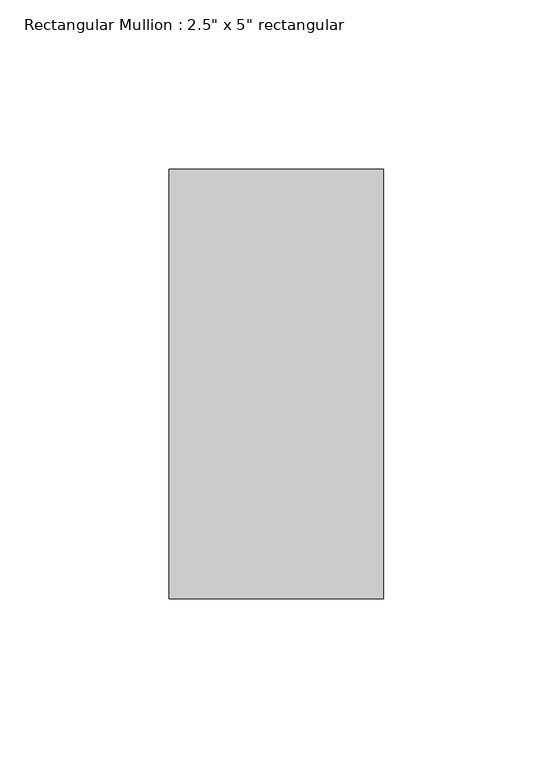
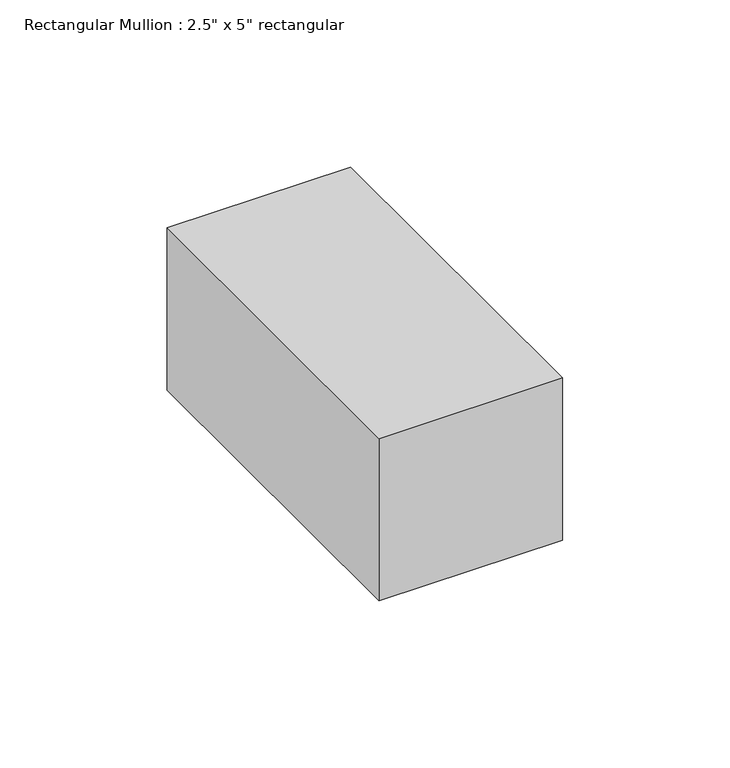
"""IFC4 building model written with IfcOpenShell, lengths in millimetres: member geometry."""

from ifc_helpers import new_model, si_unit, frame, origin, place, context, project, spatial, polyline, outline, extrude, source, transform, mapped, element, save


def member_4557678a(model_context):
    return source(origin(), model_context, "Body", "SweptSolid", [
        extrude(outline(polyline([(31.75, 63.5), (31.75, -63.5), (-31.75, -63.5), (-31.75, 63.5), (31.75, 63.5)])), frame((0.0, 0.0, -59.2666667), z_axis=(0.0, 0.0, 1.0), x_axis=(1.0, 0.0, 0.0)), (0.0, 0.0, 1.0), 59.2666667),
    ])


if __name__ == "__main__":
    model = new_model("IFC4")
    model_context = context("Model", 3, world=origin())
    ifc_project = project(units=[si_unit("LENGTHUNIT", "METRE", prefix="MILLI")], contexts=[model_context])
    site = spatial("IfcSite", under=ifc_project)
    building = spatial("IfcBuilding", under=site)
    placement = place(None, origin())
    member_shape = member_4557678a(model_context)
    element("IfcMember", 1, ObjectType="Rectangular Mullion : 2.5\" x 5\" rectangular", at=placement, inside=building, context=model_context, shape_type="MappedRepresentation", body=[
        mapped(member_shape, transform((0.0, 0.0, 0.0), x_axis=(1.0, 0.0, 0.0), y_axis=(0.0, 1.0, 0.0), z_axis=(0.0, 0.0, 1.0))),
    ])
    save(model, "model.ifc")

# Revit data of these elements
# Type "Rectangular Mullion : 2.5\" x 5\" rectangular"
#   built-in parameter 1007304 = 0.416667 (stored number, unit not read)
#   built-in parameter 1007301 = 0.104167 (stored number, unit not read)
#   built-in parameter 1007300 = 0.104167 (stored number, unit not read)
# Element 1 (IfcMember, "Rectangular Mullion : 2.5\" x 5\" rectangular")
#   Materials on its faces: "Aluminum"
# Materials
#   "Aluminum": class "Metal", colour RGB 247 247 247, transparency 0, Description = "Aluminum 6061", Cost = 0
